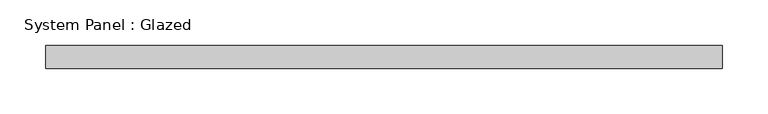
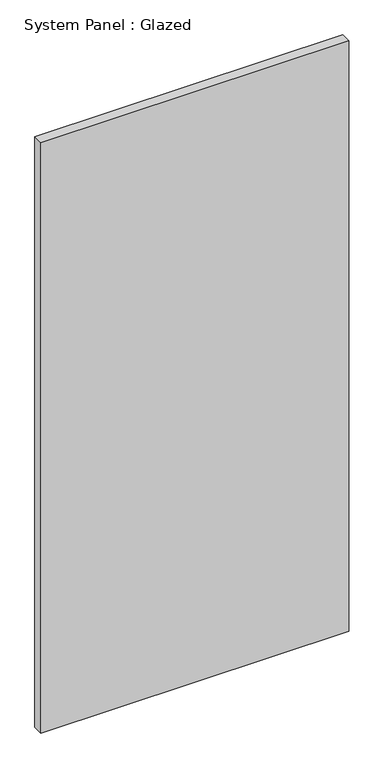
"""IFC4 building model written with IfcOpenShell, lengths in millimetres: plate geometry, System Panel : Glazed."""

from ifc_helpers import new_model, si_unit, origin, origin_with_axes, place, context, project, spatial, polyline, outline, extrude, source, transform, mapped, element, save


def system_panel_glazed_822919b4(model_context):
    return source(origin(), model_context, "Body", "SweptSolid", [
        extrude(outline(polyline([(371.475, 19.05), (-371.475, 19.05), (-371.475, 44.45), (371.475, 44.45), (371.475, 19.05)])), origin_with_axes(), (0.0, 0.0, 1.0), 1506.9367938),
    ])


if __name__ == "__main__":
    model = new_model("IFC4")
    model_context = context("Model", 3, world=origin())
    ifc_project = project(units=[si_unit("LENGTHUNIT", "METRE", prefix="MILLI")], contexts=[model_context])
    site = spatial("IfcSite", under=ifc_project)
    building = spatial("IfcBuilding", under=site)
    placement = place(None, origin())
    system_panel_glazed_shape = system_panel_glazed_822919b4(model_context)
    element("IfcPlate", 1, ObjectType="System Panel : Glazed", at=placement, inside=building, context=model_context, shape_type="MappedRepresentation", body=[
        mapped(system_panel_glazed_shape, transform((0.0, 0.0, 0.0), x_axis=(1.0, 0.0, 0.0), y_axis=(0.0, 1.0, 0.0), z_axis=(0.0, 0.0, 1.0))),
    ])
    save(model, "model.ifc")

# Revit data of these elements
# Type "System Panel : Glazed"
#   Construction Type Id = "GSP4R"
#   Analytic Construction = "1/8 in Pilkington single glazing"
#   Visual Light Transmittance = 0.9
#   Solar Heat Gain Coefficient = 0.86
#   Heat Transfer Coefficient (U) = 1.18115 BTU/(h·ft²·°F)
#   Define Thermal Properties by = 1
# Element 1 (IfcPlate, "System Panel : Glazed")
#   Materials on its faces: "Glass"
# Materials
#   "Glass": class "Glass", colour RGB 0 128 192, transparency 0.75, Description = "Soda Lime Glass", Cost = 0
